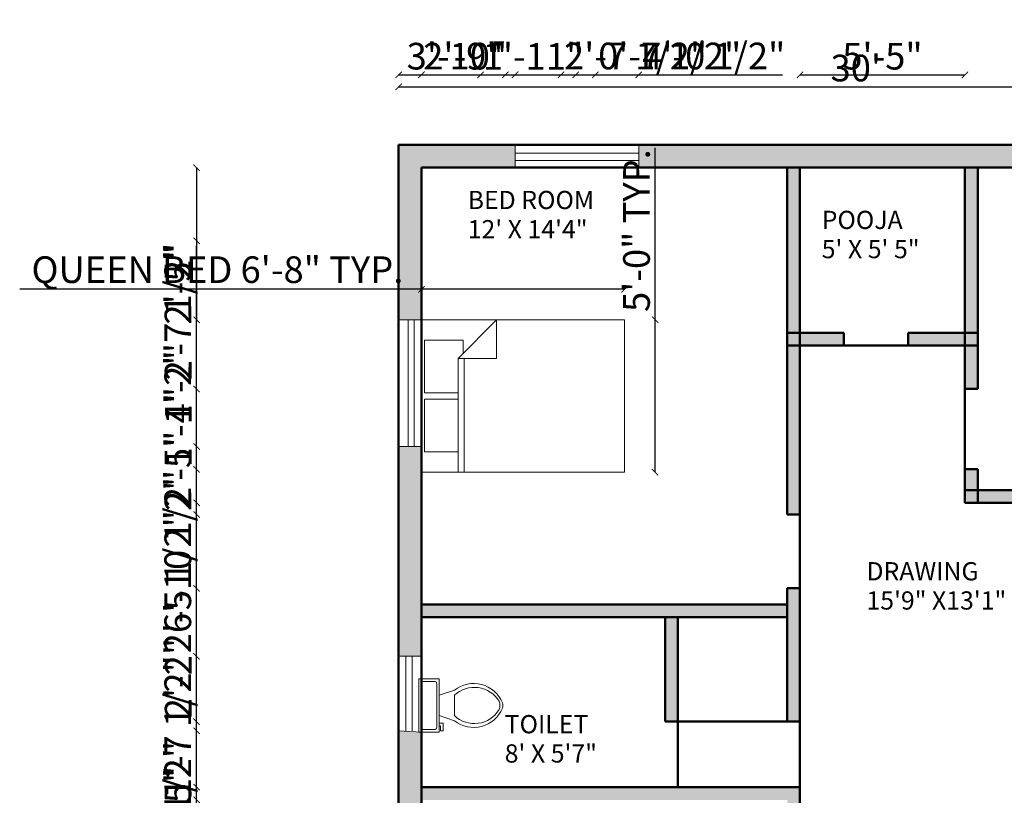
# Model space of a CAD drawing. Units: inches. Extents: x 1699 to 2290, y 1404 to 1978.
# Tile 2 of 4: x 1699 to 2086, y 1665 to 1971. Entities that reach past the tile are written whole.
import ezdxf

# ---------------------------------------------------------------- set-up
doc = ezdxf.new("R2010")
doc.units = ezdxf.units.IN
for name, color, linetype, lineweight in [('A-ANNO-DIMS', 2, 'Continuous', 18), ('A-AREA-IDEN', 7, 'Continuous', 25), ('A-FLOR-FIXT', 9, 'Continuous', 18), ('A-FURN', 8, 'Continuous', 18), ('A-WALL', 7, 'Continuous', 50), ('A-WALL-PATT', 17, 'Continuous', 13), ('window', 3, 'Continuous', 18)]:
    doc.layers.add(name, color=color, linetype=linetype, lineweight=lineweight)
doc.styles.get("Standard").update_dxf_attribs({"font": 'arial.ttf'})
doc.dimstyles.new('ISO-25', dxfattribs={"dimtxt": 10.5, "dimasz": 2.5, "dimexe": 1.25, "dimexo": 0.625, "dimtad": 1, "dimdec": 0, "dimlunit": 4, "dimtxsty": 'Standard', "dimblk": 'ARCHTICK', "dimcen": 2.5, "dimse1": 1, "dimse2": 1, "dimclrd": 4, "dimclrt": 2, "dimadec": 0, "dimazin": 0, "dimtfac": 1, "dimtdec": 0, "dimtmove": 0, "dimatfit": 3, "dimfxl": 1, "dimarcsym": 0})

# ---------------------------------------------------------------- blocks, each defined once
blk = doc.blocks.new('*U3')
for p, q in [((9.5, -6), (9.5, -2)), ((-10, -8.5), (-8, -8.5)), ((-10, -9.5), (-10, -8.5)), ((-7, -9.5), (-10, -9.5)), ((-8, -8.5), (-8, -8)), ((-7, -8), (-7, -9.5)), ((-4, -8), (-6, -14)), ((4, -8), (6, -14)), ((4, -14), (-4, -14))]:
    blk.add_line(p, q)
blk.add_lwpolyline([(10.5, -8), (10.5, 0), (-10.5, 0), (-10.5, -8)], close=True)
for points in [[(-9.5, -2), (-9.5, -6)], [(8.5, -1), (-8.5, -1)], [(-8.5, -7), (8.5, -7)]]:
    blk.add_lwpolyline(points)
for centre, radius, start, end in [((-8.62, -1.88), 0.884, 81.8699, 188.1301), ((8.62, -1.88), 0.884, 351.8699, 98.1301), ((-8.62, -6.12), 0.884, 171.8699, 278.1301), ((8.62, -6.12), 0.884, 261.8699, 8.1301), ((3.52, -21.58), 12.17, 141.4691, 247.9714), ((4.2, -21.82), 11.33, 136.3677, 238.9468), ((-3.52, -21.58), 12.17, 292.0284, 38.5307), ((-4.2, -21.82), 11.33, 301.053, 43.6321), ((0, -27.88), 4, 245.7318, 294.2682), ((0, -29), 4, 254.8605, 285.1395)]:
    blk.add_arc(centre, radius, start, end)
blk = doc.blocks.new('Bed - Queen')
for p, q in [((0, -80.00003), (0, 0)), ((0, 0), (59.99999, 0)), ((59.99999, 0), (59.99999, -80.00003)), ((7.99999, -1.2), (28.79998, -1.2)), ((7.99999, -14.4), (7.99999, -1.2)), ((28.79998, -1.2), (28.79998, -14.4)), ((31.19999, -1.2), (51.99999, -1.2)), ((31.19999, -14.4), (31.19999, -1.2)), ((51.99999, -1.2), (51.99999, -16.4)), ((0, -14.4), (44.8, -14.4)), ((59.99999, -29.6), (44.8, -14.4)), ((44.8, -14.4), (44.8, -29.6)), ((44.8, -16.8), (0, -16.8)), ((51.99999, -16.4), (46.79936, -16.4)), ((44.8, -29.6), (59.99999, -29.6)), ((59.99999, -80.00003), (0, -80.00003))]:
    blk.add_line(p, q)
blk = doc.blocks.new('_ArchTick')
at = {"color": 0, "linetype": 'ByBlock', "const_width": 0.15}
blk.add_lwpolyline([(-0.5, -0.5), (0.5, 0.5)], dxfattribs=at)
blk = doc.blocks.new('*D10')
at = {"layer": 'A-ANNO-DIMS', "color": 0, "lineweight": -2, "transparency": 16777216}
blk.add_line((1847.82, 1944.45), (2207.82, 1944.45), dxfattribs=at)
at = {"layer": 'Defpoints', "color": 0, "transparency": 16777216}
for p in [(2207.82, 1944.45), (1847.82, 1921.58), (2207.82, 1921.58)]:
    blk.add_point(p, dxfattribs=at)
at = {"layer": 'A-ANNO-DIMS', "color": 0, "lineweight": -2, "transparency": 16777216, "xscale": 2.5, "yscale": 2.5, "zscale": 2.5, "rotation": 180}
blk.add_blockref('_ArchTick', (1847.82, 1944.45), dxfattribs=at)
at = {"layer": 'A-ANNO-DIMS', "color": 0, "lineweight": -2, "transparency": 16777216, "xscale": 2.5, "yscale": 2.5, "zscale": 2.5}
blk.add_blockref('_ArchTick', (2207.82, 1944.45), dxfattribs=at)
at = {"layer": 'A-ANNO-DIMS', "color": 0, "transparency": 16777216, "insert": (2027.82, 1950.44), "char_height": 10.5, "attachment_point": 5}
blk.add_mtext("30'", dxfattribs=at)
blk = doc.blocks.new('*D12')
at = {"layer": 'A-ANNO-DIMS', "color": 4, "lineweight": -2, "transparency": 16777216}
for p, q in [((1856.82, 1864.66), (1698.62, 1864.66)), ((1936.82, 1864.66), (1856.82, 1864.66))]:
    blk.add_line(p, q, dxfattribs=at)
at = {"layer": 'Defpoints', "color": 0, "transparency": 16777216}
for p in [(1856.82, 1864.66), (1856.82, 1852.66), (1936.82, 1852.66)]:
    blk.add_point(p, dxfattribs=at)
at = {"layer": 'A-ANNO-DIMS', "color": 4, "lineweight": -2, "transparency": 16777216, "xscale": 2.5, "yscale": 2.5, "zscale": 2.5, "rotation": 180}
blk.add_blockref('_ArchTick', (1856.82, 1864.66), dxfattribs=at)
at = {"layer": 'A-ANNO-DIMS', "color": 4, "lineweight": -2, "transparency": 16777216, "xscale": 2.5, "yscale": 2.5, "zscale": 2.5}
blk.add_blockref('_ArchTick', (1936.82, 1864.66), dxfattribs=at)
at = {"layer": 'A-ANNO-DIMS', "color": 2, "transparency": 16777216, "insert": (1776.47, 1871.04), "char_height": 10.5, "attachment_point": 5}
blk.add_mtext('QUEEN BED 6\'-8" TYP.', dxfattribs=at)
blk = doc.blocks.new('*D13')
at = {"layer": 'A-ANNO-DIMS', "color": 4, "lineweight": -2, "transparency": 16777216}
for p, q in [((1948.82, 1852.66), (1948.82, 1920.42)), ((1948.82, 1792.66), (1948.82, 1852.66))]:
    blk.add_line(p, q, dxfattribs=at)
at = {"layer": 'Defpoints', "color": 0, "transparency": 16777216}
for p in [(1936.82, 1852.66), (1948.82, 1852.66), (1936.82, 1792.66)]:
    blk.add_point(p, dxfattribs=at)
at = {"layer": 'A-ANNO-DIMS', "color": 4, "lineweight": -2, "transparency": 16777216, "xscale": 2.5, "yscale": 2.5, "zscale": 2.5}
for p, rotation in [((1948.82, 1852.66), 90), ((1948.82, 1792.66), 270)]:
    blk.add_blockref('_ArchTick', p, dxfattribs=dict(at, rotation=rotation))
at = {"layer": 'A-ANNO-DIMS', "color": 2, "transparency": 16777216, "insert": (1942.84, 1887.79), "char_height": 10.5, "attachment_point": 5, "rotation": 90}
blk.add_mtext('5\'-0" TYP.', dxfattribs=at)
blk = doc.blocks.new('*D27')
at = {"layer": 'A-ANNO-DIMS', "color": 4, "lineweight": -2, "transparency": 16777216}
blk.add_line((2005.82, 1949.13), (2070.82, 1949.13), dxfattribs=at)
at = {"layer": 'Defpoints', "color": 0, "transparency": 16777216}
for p in [(2070.82, 1949.13), (2005.82, 1450.58), (2070.82, 1450.58)]:
    blk.add_point(p, dxfattribs=at)
at = {"layer": 'A-ANNO-DIMS', "color": 4, "lineweight": -2, "transparency": 16777216, "xscale": 2.5, "yscale": 2.5, "zscale": 2.5, "rotation": 180}
blk.add_blockref('_ArchTick', (2005.82, 1949.13), dxfattribs=at)
at = {"layer": 'A-ANNO-DIMS', "color": 4, "lineweight": -2, "transparency": 16777216, "xscale": 2.5, "yscale": 2.5, "zscale": 2.5}
blk.add_blockref('_ArchTick', (2070.82, 1949.13), dxfattribs=at)
at = {"layer": 'A-ANNO-DIMS', "color": 2, "transparency": 16777216, "insert": (2038.32, 1955.1), "char_height": 10.5, "attachment_point": 5}
blk.add_mtext('5\'-5"', dxfattribs=at)
blk = doc.blocks.new('*D32')
at = {"layer": 'A-ANNO-DIMS', "color": 4, "lineweight": -2, "transparency": 16777216}
blk.add_line((1768.27, 1626.46), (1768.27, 1690.77), dxfattribs=at)
at = {"layer": 'Defpoints', "color": 0, "transparency": 16777216}
for p in [(1768.27, 1690.77), (1847.82, 1690.77), (1847.82, 1626.46)]:
    blk.add_point(p, dxfattribs=at)
at = {"layer": 'A-ANNO-DIMS', "color": 4, "lineweight": -2, "transparency": 16777216, "xscale": 2.5, "yscale": 2.5, "zscale": 2.5}
for p, rotation in [((1768.27, 1690.77), 90), ((1768.27, 1626.46), 270)]:
    blk.add_blockref('_ArchTick', p, dxfattribs=dict(at, rotation=rotation))
at = {"layer": 'A-ANNO-DIMS', "color": 2, "transparency": 16777216, "insert": (1762.22, 1658.62), "char_height": 10.5, "attachment_point": 5, "rotation": 90}
blk.add_mtext('5\'-4 1/2"', dxfattribs=at)
blk = doc.blocks.new('*D33')
at = {"layer": 'A-ANNO-DIMS', "color": 4, "lineweight": -2, "transparency": 16777216}
for p, q in [((1768.27, 1720.13), (1768.27, 1776.43)), ((1768.27, 1690.77), (1768.27, 1720.13))]:
    blk.add_line(p, q, dxfattribs=at)
at = {"layer": 'Defpoints', "color": 0, "transparency": 16777216}
for p in [(1768.27, 1720.13), (1847.82, 1720.13), (1847.82, 1690.77)]:
    blk.add_point(p, dxfattribs=at)
at = {"layer": 'A-ANNO-DIMS', "color": 4, "lineweight": -2, "transparency": 16777216, "xscale": 2.5, "yscale": 2.5, "zscale": 2.5}
for p, rotation in [((1768.27, 1720.13), 90), ((1768.27, 1690.77), 270)]:
    blk.add_blockref('_ArchTick', p, dxfattribs=dict(at, rotation=rotation))
at = {"layer": 'A-ANNO-DIMS', "color": 2, "transparency": 16777216, "insert": (1762.22, 1749.53), "char_height": 10.5, "attachment_point": 5, "rotation": 90}
blk.add_mtext('2\'-5 1/2"', dxfattribs=at)
blk = doc.blocks.new('*D34')
at = {"layer": 'A-ANNO-DIMS', "color": 4, "lineweight": -2, "transparency": 16777216}
blk.add_line((1768.27, 1720.13), (1768.27, 1802.75), dxfattribs=at)
at = {"layer": 'Defpoints', "color": 0, "transparency": 16777216}
for p in [(1768.27, 1802.75), (1847.82, 1802.75), (1847.82, 1720.13)]:
    blk.add_point(p, dxfattribs=at)
at = {"layer": 'A-ANNO-DIMS', "color": 4, "lineweight": -2, "transparency": 16777216, "xscale": 2.5, "yscale": 2.5, "zscale": 2.5}
for p, rotation in [((1768.27, 1802.75), 90), ((1768.27, 1720.13), 270)]:
    blk.add_blockref('_ArchTick', p, dxfattribs=dict(at, rotation=rotation))
at = {"layer": 'A-ANNO-DIMS', "color": 2, "transparency": 16777216, "insert": (1762.22, 1761.44), "char_height": 10.5, "attachment_point": 5, "rotation": 90}
blk.add_mtext('6\'-10 1/2"', dxfattribs=at)
blk = doc.blocks.new('*D35')
at = {"layer": 'A-ANNO-DIMS', "color": 4, "lineweight": -2, "transparency": 16777216}
blk.add_line((1768.27, 1802.75), (1768.27, 1852.66), dxfattribs=at)
at = {"layer": 'Defpoints', "color": 0, "transparency": 16777216}
for p in [(1768.27, 1852.66), (1847.82, 1852.66), (1847.82, 1802.75)]:
    blk.add_point(p, dxfattribs=at)
at = {"layer": 'A-ANNO-DIMS', "color": 4, "lineweight": -2, "transparency": 16777216, "xscale": 2.5, "yscale": 2.5, "zscale": 2.5}
for p, rotation in [((1768.27, 1852.66), 90), ((1768.27, 1802.75), 270)]:
    blk.add_blockref('_ArchTick', p, dxfattribs=dict(at, rotation=rotation))
at = {"layer": 'A-ANNO-DIMS', "color": 2, "transparency": 16777216, "insert": (1762.38, 1827.71), "char_height": 10.5, "attachment_point": 5, "rotation": 90}
blk.add_mtext('4\'-2"', dxfattribs=at)
blk = doc.blocks.new('*D41')
at = {"layer": 'A-ANNO-DIMS', "color": 4, "lineweight": -2, "transparency": 16777216}
for p, q in [((1768.27, 1825.42), (1768.27, 1881.73)), ((1768.27, 1793.79), (1768.27, 1825.42))]:
    blk.add_line(p, q, dxfattribs=at)
at = {"layer": 'Defpoints', "color": 0, "transparency": 16777216}
for p in [(1768.27, 1825.42), (2075.82, 1825.42), (2075.82, 1793.79)]:
    blk.add_point(p, dxfattribs=at)
at = {"layer": 'A-ANNO-DIMS', "color": 4, "lineweight": -2, "transparency": 16777216, "xscale": 2.5, "yscale": 2.5, "zscale": 2.5}
for p, rotation in [((1768.27, 1825.42), 90), ((1768.27, 1793.79), 270)]:
    blk.add_blockref('_ArchTick', p, dxfattribs=dict(at, rotation=rotation))
at = {"layer": 'A-ANNO-DIMS', "color": 2, "transparency": 16777216, "insert": (1762.22, 1854.83), "char_height": 10.5, "attachment_point": 5, "rotation": 90}
blk.add_mtext('2\'-7 1/2"', dxfattribs=at)
blk = doc.blocks.new('*D43')
at = {"layer": 'A-ANNO-DIMS', "color": 4, "lineweight": -2, "transparency": 16777216}
for p, q in [((1768.27, 1912.58), (1768.27, 1883.78)), ((1768.27, 1883.78), (1768.27, 1851.94))]:
    blk.add_line(p, q, dxfattribs=at)
at = {"layer": 'Defpoints', "color": 0, "transparency": 16777216}
for p in [(2103.12, 1912.58), (1768.27, 1883.78), (2103.12, 1883.78)]:
    blk.add_point(p, dxfattribs=at)
at = {"layer": 'A-ANNO-DIMS', "color": 4, "lineweight": -2, "transparency": 16777216, "xscale": 2.5, "yscale": 2.5, "zscale": 2.5}
for p, rotation in [((1768.27, 1912.58), 90), ((1768.27, 1883.78), 270)]:
    blk.add_blockref('_ArchTick', p, dxfattribs=dict(at, rotation=rotation))
at = {"layer": 'A-ANNO-DIMS', "color": 2, "transparency": 16777216, "insert": (1762.29, 1866.61), "char_height": 10.5, "attachment_point": 5, "rotation": 90}
blk.add_mtext('2\'-5"', dxfattribs=at)
blk = doc.blocks.new('*D44')
at = {"layer": 'A-ANNO-DIMS', "color": 4, "lineweight": -2, "transparency": 16777216}
blk.add_line((1847.82, 1949.13), (1893.7, 1949.13), dxfattribs=at)
at = {"layer": 'Defpoints', "color": 0, "transparency": 16777216}
for p in [(1893.7, 1949.13), (1847.82, 1921.58), (1893.7, 1921.58)]:
    blk.add_point(p, dxfattribs=at)
at = {"layer": 'A-ANNO-DIMS', "color": 4, "lineweight": -2, "transparency": 16777216, "xscale": 2.5, "yscale": 2.5, "zscale": 2.5, "rotation": 180}
blk.add_blockref('_ArchTick', (1847.82, 1949.13), dxfattribs=at)
at = {"layer": 'A-ANNO-DIMS', "color": 4, "lineweight": -2, "transparency": 16777216, "xscale": 2.5, "yscale": 2.5, "zscale": 2.5}
blk.add_blockref('_ArchTick', (1893.7, 1949.13), dxfattribs=at)
at = {"layer": 'A-ANNO-DIMS', "color": 2, "transparency": 16777216, "insert": (1870.76, 1955.12), "char_height": 10.5, "attachment_point": 5}
blk.add_mtext('3\'-10"', dxfattribs=at)
blk = doc.blocks.new('*D45')
at = {"layer": 'A-ANNO-DIMS', "color": 4, "lineweight": -2, "transparency": 16777216}
for p, q in [((1893.7, 1949.13), (1942.38, 1949.13)), ((1942.38, 1949.13), (1998.93, 1949.13))]:
    blk.add_line(p, q, dxfattribs=at)
at = {"layer": 'Defpoints', "color": 0, "transparency": 16777216}
for p in [(1942.38, 1949.13), (1893.7, 1921.58), (1942.38, 1921.58)]:
    blk.add_point(p, dxfattribs=at)
at = {"layer": 'A-ANNO-DIMS', "color": 4, "lineweight": -2, "transparency": 16777216, "xscale": 2.5, "yscale": 2.5, "zscale": 2.5, "rotation": 180}
blk.add_blockref('_ArchTick', (1893.7, 1949.13), dxfattribs=at)
at = {"layer": 'A-ANNO-DIMS', "color": 4, "lineweight": -2, "transparency": 16777216, "xscale": 2.5, "yscale": 2.5, "zscale": 2.5}
blk.add_blockref('_ArchTick', (1942.38, 1949.13), dxfattribs=at)
at = {"layer": 'A-ANNO-DIMS', "color": 2, "transparency": 16777216, "insert": (1971.9, 1955.19), "char_height": 10.5, "attachment_point": 5}
blk.add_mtext('4\'-0 1/2"', dxfattribs=at)
blk = doc.blocks.new('*D50')
at = {"layer": 'A-ANNO-DIMS', "color": 4, "lineweight": -2, "transparency": 16777216}
for p, q in [((1768.27, 1776.01), (1768.27, 1807.85)), ((1768.27, 1746.92), (1768.27, 1776.01))]:
    blk.add_line(p, q, dxfattribs=at)
at = {"layer": 'Defpoints', "color": 0, "transparency": 16777216}
for p in [(1768.27, 1776.01), (2000.82, 1776.01), (2000.82, 1746.92)]:
    blk.add_point(p, dxfattribs=at)
at = {"layer": 'A-ANNO-DIMS', "color": 4, "lineweight": -2, "transparency": 16777216, "xscale": 2.5, "yscale": 2.5, "zscale": 2.5}
for p, rotation in [((1768.27, 1776.01), 90), ((1768.27, 1746.92), 270)]:
    blk.add_blockref('_ArchTick', p, dxfattribs=dict(at, rotation=rotation))
at = {"layer": 'A-ANNO-DIMS', "color": 2, "transparency": 16777216, "insert": (1762.29, 1793.18), "char_height": 10.5, "attachment_point": 5, "rotation": 90}
blk.add_mtext('2\'-5"', dxfattribs=at)
blk = doc.blocks.new('*D51')
at = {"layer": 'A-ANNO-DIMS', "color": 4, "lineweight": -2, "transparency": 16777216}
for p, q in [((1768.27, 1644.06), (1768.27, 1675.9)), ((1768.27, 1615.11), (1768.27, 1644.06))]:
    blk.add_line(p, q, dxfattribs=at)
at = {"layer": 'Defpoints', "color": 0, "transparency": 16777216}
for p in [(1768.27, 1644.06), (2000.82, 1644.06), (2000.82, 1615.11)]:
    blk.add_point(p, dxfattribs=at)
at = {"layer": 'A-ANNO-DIMS', "color": 4, "lineweight": -2, "transparency": 16777216, "xscale": 2.5, "yscale": 2.5, "zscale": 2.5}
for p, rotation in [((1768.27, 1644.06), 90), ((1768.27, 1615.11), 270)]:
    blk.add_blockref('_ArchTick', p, dxfattribs=dict(at, rotation=rotation))
at = {"layer": 'A-ANNO-DIMS', "color": 2, "transparency": 16777216, "insert": (1762.29, 1661.23), "char_height": 10.5, "attachment_point": 5, "rotation": 90}
blk.add_mtext('2\'-5"', dxfattribs=at)
blk = doc.blocks.new('*D52')
at = {"layer": 'A-ANNO-DIMS', "color": 4, "lineweight": -2, "transparency": 16777216}
for p, q in [((2023.18, 1414.03), (2048.43, 1414.03)), ((2048.43, 1414.03), (2080.27, 1414.03))]:
    blk.add_line(p, q, dxfattribs=at)
at = {"layer": 'Defpoints', "color": 0, "transparency": 16777216}
for p in [(2023.18, 1842.58), (2048.43, 1842.58), (2048.43, 1414.03)]:
    blk.add_point(p, dxfattribs=at)
at = {"layer": 'A-ANNO-DIMS', "color": 4, "lineweight": -2, "transparency": 16777216, "xscale": 2.5, "yscale": 2.5, "zscale": 2.5, "rotation": 180}
blk.add_blockref('_ArchTick', (2023.18, 1414.03), dxfattribs=at)
at = {"layer": 'A-ANNO-DIMS', "color": 4, "lineweight": -2, "transparency": 16777216, "xscale": 2.5, "yscale": 2.5, "zscale": 2.5}
blk.add_blockref('_ArchTick', (2048.43, 1414.03), dxfattribs=at)
at = {"layer": 'A-ANNO-DIMS', "color": 2, "transparency": 16777216, "insert": (2065.6, 1419.93), "char_height": 10.5, "attachment_point": 5}
blk.add_mtext('2\'-1"', dxfattribs=at)
blk = doc.blocks.new('*D54')
at = {"layer": 'A-ANNO-DIMS', "color": 4, "lineweight": -2, "transparency": 16777216}
for p, q in [((1768.27, 1694.4), (1768.27, 1726.24)), ((1768.27, 1668.58), (1768.27, 1694.4))]:
    blk.add_line(p, q, dxfattribs=at)
at = {"layer": 'Defpoints', "color": 0, "transparency": 16777216}
for p in [(1768.27, 1694.4), (2005.82, 1694.4), (2005.82, 1668.58)]:
    blk.add_point(p, dxfattribs=at)
at = {"layer": 'A-ANNO-DIMS', "color": 4, "lineweight": -2, "transparency": 16777216, "xscale": 2.5, "yscale": 2.5, "zscale": 2.5}
for p, rotation in [((1768.27, 1694.4), 90), ((1768.27, 1668.58), 270)]:
    blk.add_blockref('_ArchTick', p, dxfattribs=dict(at, rotation=rotation))
at = {"layer": 'A-ANNO-DIMS', "color": 2, "transparency": 16777216, "insert": (1762.38, 1711.57), "char_height": 10.5, "attachment_point": 5, "rotation": 90}
blk.add_mtext('2\'-2"', dxfattribs=at)
blk = doc.blocks.new('*D56')
at = {"layer": 'A-ANNO-DIMS', "color": 4, "lineweight": -2, "transparency": 16777216}
for p, q in [((1880.06, 1949.13), (1911.72, 1949.13)), ((1911.72, 1949.13), (1968.03, 1949.13))]:
    blk.add_line(p, q, dxfattribs=at)
at = {"layer": 'Defpoints', "color": 0, "transparency": 16777216}
for p in [(1911.72, 1949.13), (1880.06, 1519.58), (1911.72, 1519.58)]:
    blk.add_point(p, dxfattribs=at)
at = {"layer": 'A-ANNO-DIMS', "color": 4, "lineweight": -2, "transparency": 16777216, "xscale": 2.5, "yscale": 2.5, "zscale": 2.5, "rotation": 180}
blk.add_blockref('_ArchTick', (1880.06, 1949.13), dxfattribs=at)
at = {"layer": 'A-ANNO-DIMS', "color": 4, "lineweight": -2, "transparency": 16777216, "xscale": 2.5, "yscale": 2.5, "zscale": 2.5}
blk.add_blockref('_ArchTick', (1911.72, 1949.13), dxfattribs=at)
at = {"layer": 'A-ANNO-DIMS', "color": 2, "transparency": 16777216, "insert": (1941.12, 1955.19), "char_height": 10.5, "attachment_point": 5}
blk.add_mtext('2\'-7 1/2"', dxfattribs=at)
blk = doc.blocks.new('*D57')
at = {"layer": 'A-ANNO-DIMS', "color": 4, "lineweight": -2, "transparency": 16777216}
blk.add_line((1856.82, 1949.13), (1889.82, 1949.13), dxfattribs=at)
at = {"layer": 'Defpoints', "color": 0, "transparency": 16777216}
for p in [(1889.82, 1949.13), (1856.82, 1471.58), (1889.82, 1461.08)]:
    blk.add_point(p, dxfattribs=at)
at = {"layer": 'A-ANNO-DIMS', "color": 4, "lineweight": -2, "transparency": 16777216, "xscale": 2.5, "yscale": 2.5, "zscale": 2.5, "rotation": 180}
blk.add_blockref('_ArchTick', (1856.82, 1949.13), dxfattribs=at)
at = {"layer": 'A-ANNO-DIMS', "color": 4, "lineweight": -2, "transparency": 16777216, "xscale": 2.5, "yscale": 2.5, "zscale": 2.5}
blk.add_blockref('_ArchTick', (1889.82, 1949.13), dxfattribs=at)
at = {"layer": 'A-ANNO-DIMS', "color": 2, "transparency": 16777216, "insert": (1873.32, 1955.12), "char_height": 10.5, "attachment_point": 5}
blk.add_mtext('2\'-9"', dxfattribs=at)
blk = doc.blocks.new('*D59')
at = {"layer": 'A-ANNO-DIMS', "color": 4, "lineweight": -2, "transparency": 16777216}
for p, q in [((1917.51, 1949.13), (1925.23, 1949.13)), ((1925.23, 1949.13), (1981.36, 1949.13))]:
    blk.add_line(p, q, dxfattribs=at)
at = {"layer": 'Defpoints', "color": 0, "transparency": 16777216}
for p in [(1925.23, 1949.13), (1917.51, 1514.58), (1925.23, 1514.58)]:
    blk.add_point(p, dxfattribs=at)
at = {"layer": 'A-ANNO-DIMS', "color": 4, "lineweight": -2, "transparency": 16777216, "xscale": 2.5, "yscale": 2.5, "zscale": 2.5, "rotation": 180}
blk.add_blockref('_ArchTick', (1917.51, 1949.13), dxfattribs=at)
at = {"layer": 'A-ANNO-DIMS', "color": 4, "lineweight": -2, "transparency": 16777216, "xscale": 2.5, "yscale": 2.5, "zscale": 2.5}
blk.add_blockref('_ArchTick', (1925.23, 1949.13), dxfattribs=at)
at = {"layer": 'A-ANNO-DIMS', "color": 2, "transparency": 16777216, "insert": (1954.55, 1955.19), "char_height": 10.5, "attachment_point": 5}
blk.add_mtext('0\'-7 1/2"', dxfattribs=at)
blk = doc.blocks.new('*D61')
at = {"layer": 'A-ANNO-DIMS', "color": 4, "lineweight": -2, "transparency": 16777216}
for p, q in [((2000.82, 1414.03), (2023.18, 1414.03)), ((2023.18, 1414.03), (2086.48, 1414.03))]:
    blk.add_line(p, q, dxfattribs=at)
at = {"layer": 'Defpoints', "color": 0, "transparency": 16777216}
for p in [(2000.82, 1842.58), (2023.18, 1842.58), (2023.18, 1414.03)]:
    blk.add_point(p, dxfattribs=at)
at = {"layer": 'A-ANNO-DIMS', "color": 4, "lineweight": -2, "transparency": 16777216, "xscale": 2.5, "yscale": 2.5, "zscale": 2.5, "rotation": 180}
blk.add_blockref('_ArchTick', (2000.82, 1414.03), dxfattribs=at)
at = {"layer": 'A-ANNO-DIMS', "color": 4, "lineweight": -2, "transparency": 16777216, "xscale": 2.5, "yscale": 2.5, "zscale": 2.5}
blk.add_blockref('_ArchTick', (2023.18, 1414.03), dxfattribs=at)
at = {"layer": 'A-ANNO-DIMS', "color": 2, "transparency": 16777216, "insert": (2056.08, 1420.09), "char_height": 10.5, "attachment_point": 5}
blk.add_mtext('1\'-10 1/2"', dxfattribs=at)
blk = doc.blocks.new('*D63')
at = {"layer": 'A-ANNO-DIMS', "color": 4, "lineweight": -2, "transparency": 16777216}
for p, q in [((1768.27, 1663.58), (1768.27, 1718.72)), ((1768.27, 1644.06), (1768.27, 1663.58))]:
    blk.add_line(p, q, dxfattribs=at)
at = {"layer": 'Defpoints', "color": 0, "transparency": 16777216}
for p in [(1768.27, 1663.58), (2000.82, 1663.58), (2000.82, 1644.06)]:
    blk.add_point(p, dxfattribs=at)
at = {"layer": 'A-ANNO-DIMS', "color": 4, "lineweight": -2, "transparency": 16777216, "xscale": 2.5, "yscale": 2.5, "zscale": 2.5}
for p, rotation in [((1768.27, 1663.58), 90), ((1768.27, 1644.06), 270)]:
    blk.add_blockref('_ArchTick', p, dxfattribs=dict(at, rotation=rotation))
at = {"layer": 'A-ANNO-DIMS', "color": 2, "transparency": 16777216, "insert": (1762.22, 1692.4), "char_height": 10.5, "attachment_point": 5, "rotation": 90}
blk.add_mtext('1\'-7 1/2"', dxfattribs=at)
blk = doc.blocks.new('*D64')
at = {"layer": 'A-ANNO-DIMS', "color": 4, "lineweight": -2, "transparency": 16777216}
for p, q in [((2235.37, 1746.92), (2235.37, 1803.05)), ((2235.37, 1740.58), (2235.37, 1746.92))]:
    blk.add_line(p, q, dxfattribs=at)
at = {"layer": 'Defpoints', "color": 0, "transparency": 16777216}
for p in [(2005.82, 1746.92), (2235.37, 1746.92), (2000.82, 1740.58)]:
    blk.add_point(p, dxfattribs=at)
at = {"layer": 'A-ANNO-DIMS', "color": 4, "lineweight": -2, "transparency": 16777216, "xscale": 2.5, "yscale": 2.5, "zscale": 2.5}
for p, rotation in [((2235.37, 1746.92), 90), ((2235.37, 1740.58), 270)]:
    blk.add_blockref('_ArchTick', p, dxfattribs=dict(at, rotation=rotation))
at = {"layer": 'A-ANNO-DIMS', "color": 2, "transparency": 16777216, "insert": (2229.32, 1776.24), "char_height": 10.5, "attachment_point": 5, "rotation": 90}
blk.add_mtext('0\'-6 1/2"', dxfattribs=at)
blk = doc.blocks.new('*D65')
at = {"layer": 'A-ANNO-DIMS', "color": 4, "lineweight": -2, "transparency": 16777216}
for p, q in [((1856.82, 1949.13), (1880.06, 1949.13)), ((1880.06, 1949.13), (1918.89, 1949.13))]:
    blk.add_line(p, q, dxfattribs=at)
at = {"layer": 'Defpoints', "color": 0, "transparency": 16777216}
for p in [(1880.06, 1949.13), (1856.82, 1519.58), (1880.06, 1519.58)]:
    blk.add_point(p, dxfattribs=at)
at = {"layer": 'A-ANNO-DIMS', "color": 4, "lineweight": -2, "transparency": 16777216, "xscale": 2.5, "yscale": 2.5, "zscale": 2.5, "rotation": 180}
blk.add_blockref('_ArchTick', (1856.82, 1949.13), dxfattribs=at)
at = {"layer": 'A-ANNO-DIMS', "color": 4, "lineweight": -2, "transparency": 16777216, "xscale": 2.5, "yscale": 2.5, "zscale": 2.5}
blk.add_blockref('_ArchTick', (1880.06, 1949.13), dxfattribs=at)
at = {"layer": 'A-ANNO-DIMS', "color": 2, "transparency": 16777216, "insert": (1900.72, 1955.03), "char_height": 10.5, "attachment_point": 5}
blk.add_mtext('1\'-11"', dxfattribs=at)
blk = doc.blocks.new('*D66')
at = {"layer": 'A-ANNO-DIMS', "color": 4, "lineweight": -2, "transparency": 16777216}
for p, q in [((1768.27, 1793.79), (1768.27, 1824.46)), ((1768.27, 1780.58), (1768.27, 1793.79))]:
    blk.add_line(p, q, dxfattribs=at)
at = {"layer": 'Defpoints', "color": 0, "transparency": 16777216}
for p in [(1768.27, 1793.79), (2075.82, 1793.79), (2075.82, 1780.58)]:
    blk.add_point(p, dxfattribs=at)
at = {"layer": 'A-ANNO-DIMS', "color": 4, "lineweight": -2, "transparency": 16777216, "xscale": 2.5, "yscale": 2.5, "zscale": 2.5}
for p, rotation in [((1768.27, 1793.79), 90), ((1768.27, 1780.58), 270)]:
    blk.add_blockref('_ArchTick', p, dxfattribs=dict(at, rotation=rotation))
at = {"layer": 'A-ANNO-DIMS', "color": 2, "transparency": 16777216, "insert": (1762.38, 1810.38), "char_height": 10.5, "attachment_point": 5, "rotation": 90}
blk.add_mtext('1\'-1"', dxfattribs=at)
blk = doc.blocks.new('*D67')
at = {"layer": 'A-ANNO-DIMS', "color": 4, "lineweight": -2, "transparency": 16777216}
for p, q in [((2075.82, 1414.03), (2103.12, 1414.03)), ((2103.12, 1414.03), (2159.43, 1414.03))]:
    blk.add_line(p, q, dxfattribs=at)
at = {"layer": 'Defpoints', "color": 0, "transparency": 16777216}
for p in [(2075.82, 1912.58), (2103.12, 1883.78), (2103.12, 1414.03)]:
    blk.add_point(p, dxfattribs=at)
at = {"layer": 'A-ANNO-DIMS', "color": 4, "lineweight": -2, "transparency": 16777216, "xscale": 2.5, "yscale": 2.5, "zscale": 2.5, "rotation": 180}
blk.add_blockref('_ArchTick', (2075.82, 1414.03), dxfattribs=at)
at = {"layer": 'A-ANNO-DIMS', "color": 4, "lineweight": -2, "transparency": 16777216, "xscale": 2.5, "yscale": 2.5, "zscale": 2.5}
blk.add_blockref('_ArchTick', (2103.12, 1414.03), dxfattribs=at)
at = {"layer": 'A-ANNO-DIMS', "color": 2, "transparency": 16777216, "insert": (2132.53, 1420.09), "char_height": 10.5, "attachment_point": 5}
blk.add_mtext('2\'-3 1/2"', dxfattribs=at)

msp = doc.modelspace()

# ---------------------------------------------------------------- hatches: boundary and pattern name
at = {"layer": 'A-WALL-PATT'}
h = msp.add_hatch(color=256, dxfattribs=at)
h.dxf.hatch_style = 1
h.paths.add_polyline_path([(1893.7, 1921.58), (1847.82, 1921.58), (1847.82, 1852.66), (1856.82, 1852.66), (1856.82, 1912.58), (1893.7, 1912.58)])
h.paths.add_polyline_path([(2097.62, 1921.58), (1942.38, 1921.58), (1942.38, 1912.58), (2097.62, 1912.58)])
h.paths.add_polyline_path([(2207.82, 1921.58), (2149.1, 1921.58), (2149.1, 1912.58), (2153.96, 1912.58), (2198.82, 1912.58), (2198.82, 1877.29), (2207.82, 1877.29)])
h.paths.add_polyline_path([(2207.82, 1827.84), (2198.82, 1827.84), (2198.82, 1815.84), (2198.82, 1807.65), (2198.82, 1726.54), (2207.82, 1726.54)])
h.paths.add_polyline_path([(2207.82, 1677.38), (2198.82, 1677.38), (2198.82, 1660.38), (2198.82, 1547.09), (2207.82, 1547.09)])
h.paths.add_polyline_path([(2207.82, 1478.94), (2198.82, 1478.94), (2198.82, 1450.58), (1856.82, 1450.58), (1856.82, 1454.43), (1847.82, 1454.43), (1847.82, 1441.58), (2207.82, 1441.58)])
h.paths.add_polyline_path([(1856.82, 1567.67), (1847.82, 1567.67), (1847.82, 1476), (1856.82, 1476)])
h.paths.add_polyline_path([(1856.82, 1690.28), (1855.82, 1690.28), (1855.82, 1690.33), (1847.82, 1690.77), (1847.82, 1626.46), (1856.82, 1626.46)])
h.paths.add_polyline_path([(1856.82, 1802.75), (1847.82, 1802.75), (1847.82, 1720.13), (1856.82, 1720.13)])
h.paths.add_polyline_path([(2000.82, 1740.58), (1856.82, 1740.58), (1856.82, 1735.58), (2000.82, 1735.58)])
h.paths.add_polyline_path([(2005.82, 1668.58), (2000.82, 1668.58), (1856.82, 1668.58), (1856.82, 1663.58), (2000.82, 1663.58), (2000.82, 1644.06), (2005.82, 1644.06)])
h.paths.add_polyline_path([(2005.82, 1746.92), (2000.82, 1746.92), (2000.82, 1694.4), (2005.82, 1694.4)])
h.paths.add_polyline_path([(1957.82, 1735.58), (1952.82, 1735.58), (1952.82, 1694.4), (1957.82, 1694.4)])
h.paths.add_polyline_path([(2005.82, 1842.58), (2000.82, 1842.58), (2000.82, 1776.01), (2005.82, 1776.01)])
h.paths.add_polyline_path([(2000.82, 1519.58), (1911.72, 1519.58), (1911.72, 1514.58), (2000.82, 1514.58)])
h.paths.add_polyline_path([(1880.06, 1519.58), (1856.82, 1519.58), (1856.82, 1514.58), (1880.06, 1514.58)])
h.paths.add_polyline_path([(2005.82, 1615.11), (2000.82, 1615.11), (2000.82, 1519.58), (2005.82, 1519.58)])
h.paths.add_polyline_path([(2075.82, 1586.58), (2070.82, 1586.58), (2070.82, 1450.58), (2075.82, 1450.58)])
h.paths.add_polyline_path([(2198.82, 1591.58), (2112.54, 1591.58), (2112.54, 1586.58), (2198.82, 1586.58)])
h.paths.add_polyline_path([(2075.82, 1912.58), (2070.82, 1912.58), (2070.82, 1847.58), (2075.82, 1847.58)])
h.paths.add_polyline_path([(2198.82, 1785.58), (2075.82, 1785.58), (2075.82, 1780.58), (2198.82, 1780.58)])
h.paths.add_polyline_path([(2075.82, 1842.58), (2070.82, 1842.58), (2070.82, 1825.42), (2075.82, 1825.42)])
h.paths.add_polyline_path([(2075.82, 1847.58), (2070.82, 1847.58), (2070.82, 1842.58), (2075.82, 1842.58)])
h.paths.add_polyline_path([(2070.82, 1847.58), (2048.43, 1847.58), (2048.43, 1842.58), (2070.82, 1842.58)])
h.paths.add_polyline_path([(2023.18, 1847.58), (2005.82, 1847.58), (2005.82, 1842.58), (2023.18, 1842.58)])
h.paths.add_polyline_path([(2005.82, 1912.58), (2000.82, 1912.58), (2000.82, 1847.58), (2005.82, 1847.58)])
h.paths.add_polyline_path([(2005.82, 1847.58), (2000.82, 1847.58), (2000.82, 1842.58), (2005.82, 1842.58)])
h.paths.add_polyline_path([(2075.82, 1793.79), (2070.82, 1793.79), (2070.82, 1785.58), (2075.82, 1785.58)])
h.paths.add_polyline_path([(2075.82, 1785.58), (2070.82, 1785.58), (2070.82, 1780.58), (2075.82, 1780.58)])
h.paths.add_polyline_path([(2088.5, 1836.17), (2134.05, 1836.17), (2134.05, 1847.15), (2088.5, 1847.15)], flags=9)
h.paths.add_polyline_path([(2088.47, 1847.66), (2136.12, 1847.66), (2136.12, 1858.78), (2088.47, 1858.78)], flags=9)
h.paths.add_polyline_path([(2012.58, 1874.96), (2055.33, 1874.96), (2055.33, 1885.9), (2012.58, 1885.9)], flags=9)
h.paths.add_polyline_path([(2012.55, 1886.44), (2050.21, 1886.44), (2050.21, 1897.57), (2012.55, 1897.57)], flags=9)
h.paths.add_polyline_path([(1873.22, 1882.94), (1924.28, 1882.94), (1924.28, 1893.74), (1873.22, 1893.74)], flags=9)
h.paths.add_polyline_path([(1873.17, 1894.28), (1931.39, 1894.28), (1931.39, 1905.41), (1873.17, 1905.41)], flags=9)

# ---------------------------------------------------------------- linework, layer by layer
at = {"layer": 'A-WALL'}
for p, q in [((1856.82, 1912.58), (2198.82, 1912.58)), ((1856.82, 1450.58), (1856.82, 1912.58)), ((2000.82, 1776.01), (2000.82, 1912.58)), ((2005.82, 1450.58), (2005.82, 1912.58)), ((2070.82, 1780.58), (2070.82, 1912.58)), ((2075.82, 1825.42), (2075.82, 1912.58)), ((2000.82, 1847.58), (2023.18, 1847.58)), ((2023.18, 1847.58), (2023.18, 1842.58)), ((2048.43, 1847.58), (2048.43, 1842.58)), ((2048.43, 1847.58), (2075.82, 1847.58)), ((2000.82, 1842.58), (2075.82, 1842.58)), ((2075.82, 1825.42), (2070.82, 1825.42)), ((2075.82, 1793.79), (2070.82, 1793.79)), ((2075.82, 1780.58), (2075.82, 1793.79)), ((2070.82, 1785.58), (2198.82, 1785.58)), ((2070.82, 1780.58), (2198.82, 1780.58)), ((2005.82, 1776.01), (2000.82, 1776.01)), ((2000.82, 1694.4), (2000.82, 1746.92)), ((2005.82, 1746.92), (2000.82, 1746.92)), ((1856.82, 1740.58), (2000.82, 1740.58)), ((1856.82, 1735.58), (2000.82, 1735.58)), ((1952.82, 1694.4), (1952.82, 1735.58)), ((1957.82, 1668.58), (1957.82, 1735.58)), ((1952.82, 1694.4), (2005.82, 1694.4)), ((1856.82, 1668.58), (2000.82, 1668.58)), ((2000.82, 1668.58), (2005.82, 1668.58))]:
    msp.add_line(p, q, dxfattribs=at)
msp.add_lwpolyline([(1847.82, 1921.58), (2207.82, 1921.58), (2207.82, 1441.58), (1847.82, 1441.58)], close=True, dxfattribs=at)
at = {"layer": 'window'}
for p, q in [((1893.7, 1921.58), (1893.7, 1912.58)), ((1942.38, 1921.58), (1893.7, 1921.58)), ((1942.38, 1912.58), (1942.38, 1921.58)), ((1942.38, 1918.29), (1893.7, 1918.29)), ((1942.38, 1915.43), (1893.7, 1915.43)), ((1893.7, 1912.58), (1942.38, 1912.58)), ((1942.38, 1912.58), (1893.7, 1912.58)), ((1856.82, 1852.66), (1847.82, 1852.66)), ((1847.82, 1852.66), (1847.82, 1802.75)), ((1851.51, 1852.66), (1851.51, 1802.75)), ((1853.96, 1852.66), (1853.96, 1802.75)), ((1856.82, 1802.75), (1856.82, 1852.66)), ((1856.82, 1852.66), (1856.82, 1802.75)), ((1847.82, 1802.75), (1856.82, 1802.75)), ((1856.82, 1720.13), (1847.82, 1720.13)), ((1847.82, 1720.13), (1847.82, 1690.77)), ((1850.63, 1720.13), (1850.63, 1690.77)), ((1853.18, 1720.13), (1853.18, 1690.77)), ((1856.82, 1690.28), (1856.82, 1720.13)), ((1847.82, 1690.77), (1856.82, 1690.28))]:
    msp.add_line(p, q, dxfattribs=at)

# ---------------------------------------------------------------- block references
at = {"layer": 'A-FLOR-FIXT', "rotation": 90}
msp.add_blockref('*U3', (1855.82, 1700.78), dxfattribs=at)
at = {"layer": 'A-FURN', "rotation": 90}
msp.add_blockref('Bed - Queen', (1856.82, 1792.66), dxfattribs=at)

# ---------------------------------------------------------------- texts
at = {"layer": 'A-AREA-IDEN'}
for s, height, p in [('BED ROOM', 7.167, (1875.02, 1896.26)), ('12\' X 14\'4"', 7.1668, (1875.02, 1884.75)), ('POOJA', 7.167, (2014.41, 1888.42)), ('5\' X 5\' 5"', 7.167, (2014.41, 1876.91)), ('DRAWING ', 7.167, (2032.02, 1750.05)), ('15\'9" X13\'1"', 7.1668, (2032.02, 1738.54)), ('TOILET', 7.167, (1889.59, 1689.82)), ('8\' X 5\'7"', 7.167, (1889.59, 1678.3))]:
    msp.add_text(s, height=height, dxfattribs=at).set_placement(p)

# ---------------------------------------------------------------- dimensions: what is measured, and where the dimension line sits
at = {"layer": 'A-ANNO-DIMS'}
for base, p1, p2, override, picture, middle in [((1911.72, 1949.13), (1880.06, 1519.58), (1911.72, 1519.58), {"dimdec": 1, "dimlfac": 1, "dimrnd": 0, "dimzin": 1, "dimdsep": 46, "dimlunit": 4, "dimfrac": 2}, '*D56', (1941.12, 1955.19)), ((1942.38, 1949.13), (1893.7, 1921.58), (1942.38, 1921.58), {"dimdec": 1, "dimlfac": 1, "dimrnd": 0, "dimzin": 1, "dimdsep": 46, "dimlunit": 4, "dimfrac": 2}, '*D45', (1971.9, 1955.19)), ((1925.23, 1949.13), (1917.51, 1514.58), (1925.23, 1514.58), {"dimdec": 1, "dimlfac": 1, "dimrnd": 0, "dimzin": 1, "dimdsep": 46, "dimlunit": 4, "dimfrac": 2}, '*D59', (1954.55, 1955.19)), ((1893.7, 1949.13), (1847.82, 1921.58), (1893.7, 1921.58), {"dimdec": 1, "dimlfac": 1, "dimrnd": 0, "dimzin": 1, "dimdsep": 46, "dimlunit": 4, "dimfrac": 2}, '*D44', (1870.76, 1955.12)), ((1889.82, 1949.13), (1856.82, 1471.58), (1889.82, 1461.08), {"dimdec": 1, "dimlfac": 1, "dimrnd": 0, "dimzin": 1, "dimdsep": 46, "dimlunit": 4, "dimfrac": 2}, '*D57', (1873.32, 1955.12)), ((1880.06, 1949.13), (1856.82, 1519.58), (1880.06, 1519.58), {"dimdec": 1, "dimlfac": 1, "dimrnd": 0, "dimzin": 1, "dimdsep": 46, "dimlunit": 4, "dimfrac": 2}, '*D65', (1900.72, 1955.03)), ((2070.82, 1949.13), (2005.82, 1450.58), (2070.82, 1450.58), {"dimdec": 1, "dimlfac": 1, "dimrnd": 0, "dimzin": 1, "dimdsep": 46, "dimlunit": 4, "dimfrac": 2}, '*D27', (2038.32, 1955.1)), ((2207.82, 1944.45), (1847.82, 1921.58), (2207.82, 1921.58), {"dimclrd": 0, "dimclre": 0, "dimclrt": 0}, '*D10', (2027.82, 1950.44)), ((2103.12, 1414.03), (2075.82, 1912.58), (2103.12, 1883.78), {"dimdec": 1, "dimlfac": 1, "dimrnd": 0, "dimzin": 1, "dimdsep": 46, "dimlunit": 4, "dimfrac": 2}, '*D67', (2132.53, 1420.09)), ((2023.18, 1414.03), (2000.82, 1842.58), (2023.18, 1842.58), {"dimdec": 1, "dimlfac": 1, "dimrnd": 0, "dimzin": 1, "dimdsep": 46, "dimlunit": 4, "dimfrac": 2}, '*D61', (2056.08, 1420.09)), ((2048.4251, 1414.0349), (2023.1812, 1842.5849), (2048.4251, 1842.5849), {"dimdec": 1, "dimlfac": 1, "dimrnd": 0, "dimzin": 1, "dimdsep": 46, "dimlunit": 4, "dimfrac": 2}, '*D52', (2065.5955, 1419.9314))]:
    dim = msp.add_linear_dim(base=base, p1=p1, p2=p2, dimstyle='ISO-25', override=override, dxfattribs=at)
    dim.commit()
    dim.dimension.update_dxf_attribs({"geometry": picture, "text_midpoint": middle})
for base, p1, p2, angle, text, picture, middle in [((1948.82, 1852.66), (1936.82, 1792.66), (1936.82, 1852.66), 90, '<> TYP.', '*D13', (1942.84, 1887.79)), ((1856.82, 1864.66), (1936.82, 1852.66), (1856.82, 1852.66), 180, 'QUEEN BED <> TYP.', '*D12', (1776.47, 1871.04))]:
    dim = msp.add_linear_dim(base=base, p1=p1, p2=p2, angle=angle, text=text, dimstyle='ISO-25', override={"dimdec": 1, "dimlfac": 1, "dimrnd": 0, "dimzin": 1, "dimdsep": 46, "dimlunit": 4, "dimfrac": 2}, dxfattribs=at)
    dim.commit()
    dim.dimension.update_dxf_attribs({"geometry": picture, "text_midpoint": middle})
for base, p1, p2, picture, middle in [((1768.27, 1883.78), (2103.12, 1912.58), (2103.12, 1883.78), '*D43', (1762.29, 1866.61)), ((1768.27, 1825.42), (2075.82, 1793.79), (2075.82, 1825.42), '*D41', (1762.22, 1854.83)), ((1768.27, 1852.66), (1847.82, 1802.75), (1847.82, 1852.66), '*D35', (1762.38, 1827.71)), ((1768.27, 1793.79), (2075.82, 1780.58), (2075.82, 1793.79), '*D66', (1762.38, 1810.38)), ((1768.27, 1776.01), (2000.82, 1746.92), (2000.82, 1776.01), '*D50', (1762.29, 1793.18)), ((1768.27, 1802.75), (1847.82, 1720.13), (1847.82, 1802.75), '*D34', (1762.22, 1761.44)), ((2235.37, 1746.92), (2000.82, 1740.58), (2005.82, 1746.92), '*D64', (2229.32, 1776.24)), ((1768.27, 1720.13), (1847.82, 1690.77), (1847.82, 1720.13), '*D33', (1762.22, 1749.53)), ((1768.27, 1694.4), (2005.82, 1668.58), (2005.82, 1694.4), '*D54', (1762.38, 1711.57)), ((1768.27, 1663.58), (2000.82, 1644.06), (2000.82, 1663.58), '*D63', (1762.22, 1692.4)), ((1768.27, 1690.77), (1847.82, 1626.46), (1847.82, 1690.77), '*D32', (1762.22, 1658.62)), ((1768.2716, 1644.0554), (2000.8216, 1615.11), (2000.8216, 1644.0554), '*D51', (1762.2856, 1661.2258))]:
    dim = msp.add_linear_dim(base=base, p1=p1, p2=p2, angle=90, dimstyle='ISO-25', override={"dimdec": 1, "dimlfac": 1, "dimrnd": 0, "dimzin": 1, "dimdsep": 46, "dimlunit": 4, "dimfrac": 2}, dxfattribs=at)
    dim.commit()
    dim.dimension.update_dxf_attribs({"geometry": picture, "text_midpoint": middle})

doc.saveas('drawing.dxf')
